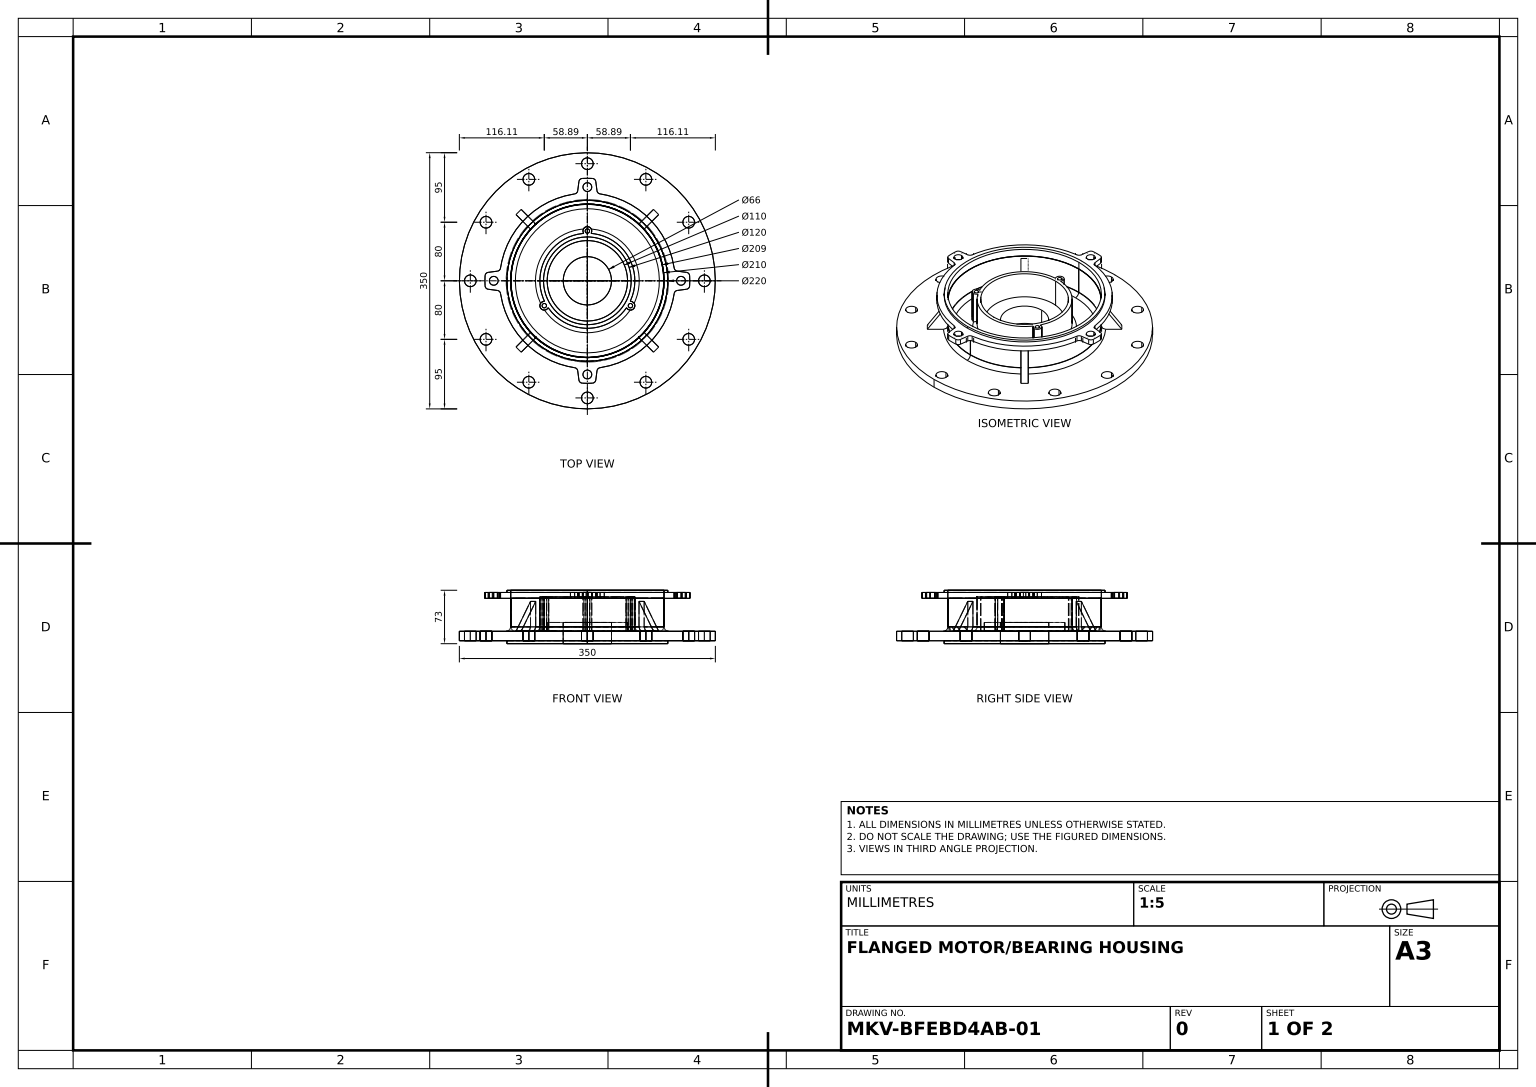
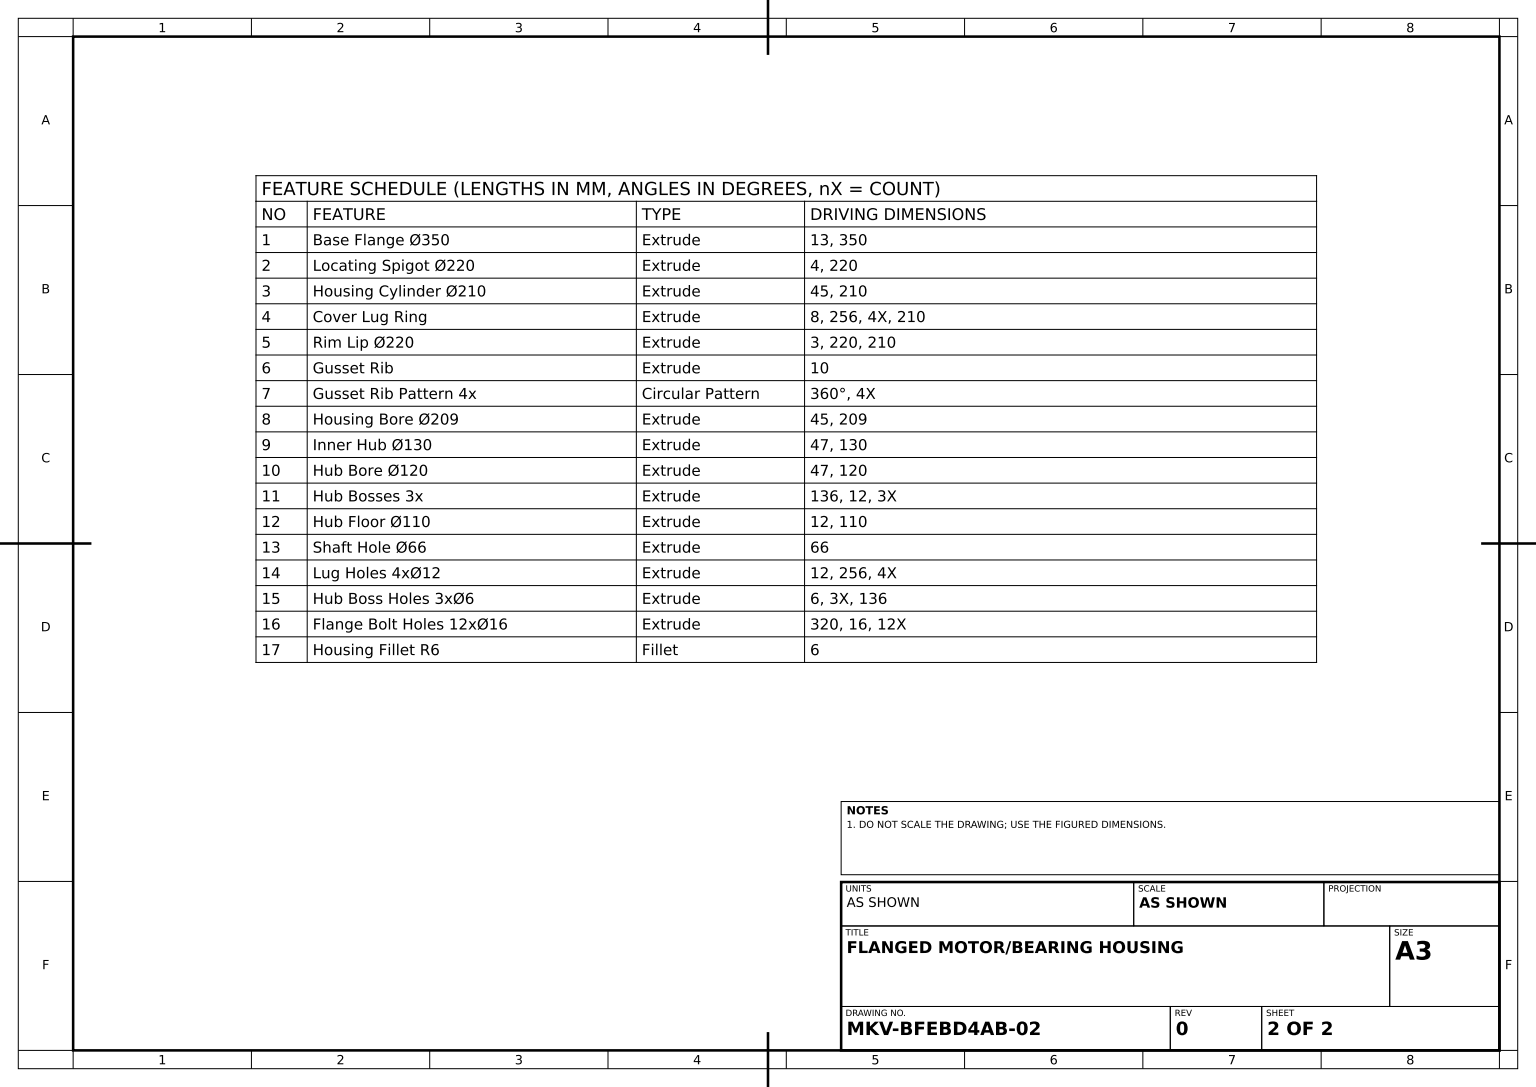
from build123d import *

# Parameters (mm, degrees)
FLANGE_SKETCH_350_R            = 175
BASE_FLANGE_350_DEPTH          = 13
SPIGOT_SKETCH_220_R            = 110
LOCATING_SPIGOT_220_DEPTH      = 4
HOUSING_SKETCH_210_R           = 105
HOUSING_CYLINDER_210_DEPTH     = 45
LUG_RING_SKETCH_R              = 105
COVER_LUG_RING_DEPTH           = 8
RIM_LIP_SKETCH_R               = 110
RIM_LIP_SKETCH_R_2             = 105
RIM_LIP_220_DEPTH              = 3
GUSSET_RIB_DEPTH               = 5
GUSSET_RIB_PATTERN_4X_COUNT    = 4
HOUSING_BORE_SKETCH_209_R      = 104.5
HOUSING_BORE_209_DEPTH         = 45
HUB_SKETCH_130_R               = 65
INNER_HUB_130_DEPTH            = 47
HUB_BORE_SKETCH_120_R          = 60
HUB_BORE_120_DEPTH             = 47
HUB_BOSSES_3X_REACH            = 257.629
HUB_BOSSES_SKETCH_3X_R         = 6
HUB_FLOOR_SKETCH_110_R         = 55
HUB_FLOOR_110_DEPTH            = 12
SHAFT_HOLE_SKETCH_66_R         = 33
SHAFT_HOLE_66_DEPTH            = 29
LUG_HOLES_SKETCH_4X_12_R       = 6
LUG_HOLES_4X_12_DEPTH          = 12
BOSS_HOLES_SKETCH_3X_6_R       = 3
HUB_BOSS_HOLES_3X_6_DEPTH      = 47
BOLT_HOLES_SKETCH_12X_16_R     = 8
FLANGE_BOLT_HOLES_12X_16_DEPTH = 13
HOUSING_FILLET_R6_R            = 6


with BuildPart() as part:
    # Flange Sketch Ø350 → Base Flange Ø350 (new body)
    with BuildSketch(Plane(origin=(0, 0, 0), x_dir=(1, 0, 0), z_dir=(0, 1, 0))):
        with Locations(Location((0, 0, 0), (0, 0, 90))):
            Circle(FLANGE_SKETCH_350_R)
    extrude(amount=BASE_FLANGE_350_DEPTH)

    # Spigot Sketch Ø220 → Locating Spigot Ø220 (add)
    with BuildSketch(Plane.XZ):
        with Locations(Location((0, 0, 0), (0, 0, 270))):
            Circle(SPIGOT_SKETCH_220_R)
    extrude(amount=LOCATING_SPIGOT_220_DEPTH)

    # Housing Sketch Ø210 → Housing Cylinder Ø210 (add)
    with BuildSketch(Plane(origin=(0, 13, 0), x_dir=(1, 0, 0), z_dir=(0, 1, 0))):
        with Locations(Location((0, 0, 0), (0, 0, 90))):
            Circle(HOUSING_SKETCH_210_R)
    extrude(amount=HOUSING_CYLINDER_210_DEPTH)

    # Gusset Rib Profile → Gusset Rib (add, symmetric)
    with BuildSketch(Plane(origin=(0, 0, 0), x_dir=(-0.707106781186549, 0, -0.7071067811865462), z_dir=(0.7071067811865462, 0, -0.707106781186549))):
        Polygon((102.938543902, 56.605912109), (102.938543902, 13), (132.938543902, 13), align=None)
    gusset_rib = extrude(amount=GUSSET_RIB_DEPTH, both=True)

    # Gusset Rib Pattern 4x: Gusset Rib ×4 about axis
    gusset_rib_pattern_4x_axis = Axis((0, 0, 0), (0, 1, 0))
    for i in range(1, GUSSET_RIB_PATTERN_4X_COUNT):
        add(gusset_rib.rotate(gusset_rib_pattern_4x_axis, i * 360 / GUSSET_RIB_PATTERN_4X_COUNT))

    # Housing Bore Sketch Ø209 → Housing Bore Ø209 (cut)
    with BuildSketch(Plane(origin=(0, 58, 0), x_dir=(1, 0, 0), z_dir=(0, 1, 0))):
        with Locations(Location((0, 0, 0), (0, 0, 270))):
            Circle(HOUSING_BORE_SKETCH_209_R)
    extrude(amount=-HOUSING_BORE_209_DEPTH, mode=Mode.SUBTRACT)

    # Hub Sketch Ø130 → Inner Hub Ø130 (add)
    with BuildSketch(Plane(origin=(0, 13, 0), x_dir=(1, 0, 0), z_dir=(0, 1, 0))):
        with Locations(Location((0, 0, 0), (0, 0, 270))):
            Circle(HUB_SKETCH_130_R)
    extrude(amount=INNER_HUB_130_DEPTH)

    # Hub Bore Sketch Ø120 → Hub Bore Ø120 (cut)
    with BuildSketch(Plane(origin=(0, 60, 0), x_dir=(1, 0, 0), z_dir=(0, 1, 0))):
        with Locations(Location((0, 0, 0), (0, 0, 270))):
            Circle(HUB_BORE_SKETCH_120_R)
    extrude(amount=-HUB_BORE_120_DEPTH, mode=Mode.SUBTRACT)

    # Hub Bosses Sketch 3x → Hub Bosses 3x (add, up to next)
    with BuildSketch(Plane(origin=(0, 60, 0), x_dir=(1, 0, 0), z_dir=(0, 1, 0)), mode=Mode.PRIVATE) as hub_bosses_3x_sk1:
        with Locations((0, 68)):
            Circle(HUB_BOSSES_SKETCH_3X_R)
    hub_bosses_3x_tool1 = extrude(hub_bosses_3x_sk1.sketch, amount=-HUB_BOSSES_3X_REACH, mode=Mode.PRIVATE) - part.part
    # Hub Bosses Sketch 3x → Hub Bosses 3x (add, up to next)
    with BuildSketch(Plane(origin=(0, 60, 0), x_dir=(1, 0, 0), z_dir=(0, 1, 0)), mode=Mode.PRIVATE) as hub_bosses_3x_sk2:
        with Locations((58.889727457, -34)):
            Circle(HUB_BOSSES_SKETCH_3X_R)
    hub_bosses_3x_tool2 = extrude(hub_bosses_3x_sk2.sketch, amount=-HUB_BOSSES_3X_REACH, mode=Mode.PRIVATE) - part.part
    # Hub Bosses Sketch 3x → Hub Bosses 3x (add, up to next)
    with BuildSketch(Plane(origin=(0, 60, 0), x_dir=(1, 0, 0), z_dir=(0, 1, 0)), mode=Mode.PRIVATE) as hub_bosses_3x_sk3:
        with Locations((-58.889727457, -34)):
            Circle(HUB_BOSSES_SKETCH_3X_R)
    hub_bosses_3x_tool3 = extrude(hub_bosses_3x_sk3.sketch, amount=-HUB_BOSSES_3X_REACH, mode=Mode.PRIVATE) - part.part
    add(hub_bosses_3x_tool1.solids().sort_by_distance((0, 60, -68))[0])
    add(hub_bosses_3x_tool2.solids().sort_by_distance((58.889727, 60, 34))[0])
    add(hub_bosses_3x_tool3.solids().sort_by_distance((-58.889727, 60, 34))[0])

    # Hub Floor Sketch Ø110 → Hub Floor Ø110 (add)
    with BuildSketch(Plane(origin=(0, 13, 0), x_dir=(1, 0, 0), z_dir=(0, 1, 0))):
        with Locations(Location((0, 0, 0), (0, 0, 270))):
            Circle(HUB_FLOOR_SKETCH_110_R)
    extrude(amount=HUB_FLOOR_110_DEPTH)

    # Shaft Hole Sketch Ø66 → Shaft Hole Ø66 (cut)
    with BuildSketch(Plane(origin=(0, 25, 0), x_dir=(1, 0, 0), z_dir=(0, 1, 0))):
        with Locations(Location((0, 0, 0), (0, 0, 270))):
            Circle(SHAFT_HOLE_SKETCH_66_R)
    extrude(amount=-SHAFT_HOLE_66_DEPTH, mode=Mode.SUBTRACT)

    # Boss Holes Sketch 3xØ6 → Hub Boss Holes 3xØ6 (cut)
    with BuildSketch(Plane(origin=(0, 60, 0), x_dir=(1, 0, 0), z_dir=(0, 1, 0))):
        with Locations(Location((0, 68, 0), (0, 0, 270))):
            Circle(BOSS_HOLES_SKETCH_3X_6_R)
        with Locations(Location((58.889727457, -34, 0), (0, 0, 270))):
            Circle(BOSS_HOLES_SKETCH_3X_6_R)
        with Locations(Location((-58.889727457, -34, 0), (0, 0, 270))):
            Circle(BOSS_HOLES_SKETCH_3X_6_R)
    extrude(amount=-HUB_BOSS_HOLES_3X_6_DEPTH, mode=Mode.SUBTRACT)

    # Bolt Holes Sketch 12xØ16 → Flange Bolt Holes 12xØ16 (cut)
    with BuildSketch(Plane(origin=(0, 13, 0), x_dir=(1, 0, 0), z_dir=(0, 1, 0))):
        with Locations(Location((0, 160, 0), (0, 0, 270))):
            Circle(BOLT_HOLES_SKETCH_12X_16_R)
        with Locations(Location((80, 138.564064606, 0), (0, 0, 270))):
            Circle(BOLT_HOLES_SKETCH_12X_16_R)
        with Locations(Location((138.564064606, 80, 0), (0, 0, 270))):
            Circle(BOLT_HOLES_SKETCH_12X_16_R)
        with Locations(Location((160, 0, 0), (0, 0, 270))):
            Circle(BOLT_HOLES_SKETCH_12X_16_R)
        with Locations(Location((138.564064606, -80, 0), (0, 0, 270))):
            Circle(BOLT_HOLES_SKETCH_12X_16_R)
        with Locations(Location((80, -138.564064606, 0), (0, 0, 270))):
            Circle(BOLT_HOLES_SKETCH_12X_16_R)
        with Locations(Location((0, -160, 0), (0, 0, 270))):
            Circle(BOLT_HOLES_SKETCH_12X_16_R)
        with Locations(Location((-80, -138.564064606, 0), (0, 0, 270))):
            Circle(BOLT_HOLES_SKETCH_12X_16_R)
        with Locations(Location((-138.564064606, -80, 0), (0, 0, 270))):
            Circle(BOLT_HOLES_SKETCH_12X_16_R)
        with Locations(Location((-160, 0, 0), (0, 0, 270))):
            Circle(BOLT_HOLES_SKETCH_12X_16_R)
        with Locations(Location((-138.564064606, 80, 0), (0, 0, 270))):
            Circle(BOLT_HOLES_SKETCH_12X_16_R)
        with Locations(Location((-80, 138.564064606, 0), (0, 0, 270))):
            Circle(BOLT_HOLES_SKETCH_12X_16_R)
    extrude(amount=-FLANGE_BOLT_HOLES_12X_16_DEPTH, mode=Mode.SUBTRACT)

    # Housing Fillet R6
    housing_fillet_r6_edges = [part.edges().sort_by_distance(p)[0] for p in [
        (56.291651246, 13, -32.5),
        (0, 13, 65),
        (-105, 13, 0),
        (0, 13, 105),
        (105, 13, 0),
        (-37.860008772, 13, -97.936815018),
        (0, 13, -104.5),
        (-56.291651246, 13, -32.5),
    ]]
    fillet(housing_fillet_r6_edges, radius=HOUSING_FILLET_R6_R)


with BuildPart() as body_2:
    # Lug Ring Sketch → Cover Lug Ring (new body)
    with BuildSketch(Plane(origin=(0, 58, 0), x_dir=(1, 0, 0), z_dir=(0, 1, 0))):
        with BuildLine():
            Line((135.492214872, 11.536480406), (123.024850581, 13.177840053))
            ThreePointArc((123.024850581, 13.177840053), (120.168019556, 14.573649393), (118.730382281, 17.409661786))
            ThreePointArc((118.730382281, 17.409661786), (84.852813742, 84.852813742), (17.409661786, 118.730382281))
            ThreePointArc((17.409661786, 118.730382281), (14.573649393, 120.168019556), (13.177840053, 123.024850581))
            Line((13.177840053, 123.024850581), (11.536480406, 135.492214872))
            ThreePointArc((11.536480406, 135.492214872), (9.96663562, 138.517308748), (6.822932251, 139.833642574))
            ThreePointArc((6.822932251, 139.833642574), (0, 140), (-6.822932251, 139.833642574))
            ThreePointArc((-6.822932251, 139.833642574), (-9.96663562, 138.517308748), (-11.536480406, 135.492214872))
            Line((-11.536480406, 135.492214872), (-13.177840053, 123.024850581))
            ThreePointArc((-13.177840053, 123.024850581), (-14.573649393, 120.168019556), (-17.409661786, 118.730382281))
            ThreePointArc((-17.409661786, 118.730382281), (-84.852813742, 84.852813742), (-118.730382281, 17.409661786))
            ThreePointArc((-118.730382281, 17.409661786), (-120.168019556, 14.573649393), (-123.024850581, 13.177840053))
            Line((-123.024850581, 13.177840053), (-135.492214872, 11.536480406))
            ThreePointArc((-135.492214872, 11.536480406), (-138.517308748, 9.96663562), (-139.833642574, 6.822932251))
            ThreePointArc((-139.833642574, 6.822932251), (-140, 0), (-139.833642574, -6.822932251))
            ThreePointArc((-139.833642574, -6.822932251), (-138.517308748, -9.96663562), (-135.492214872, -11.536480406))
            Line((-135.492214872, -11.536480406), (-123.024850581, -13.177840053))
            ThreePointArc((-123.024850581, -13.177840053), (-120.168019556, -14.573649393), (-118.730382281, -17.409661786))
            ThreePointArc((-118.730382281, -17.409661786), (-84.852813742, -84.852813742), (-17.409661786, -118.730382281))
            ThreePointArc((-17.409661786, -118.730382281), (-14.573649393, -120.168019556), (-13.177840053, -123.024850581))
            Line((-13.177840053, -123.024850581), (-11.536480406, -135.492214872))
            ThreePointArc((-11.536480406, -135.492214872), (-9.96663562, -138.517308748), (-6.822932251, -139.833642574))
            ThreePointArc((-6.822932251, -139.833642574), (0, -140), (6.822932251, -139.833642574))
            ThreePointArc((6.822932251, -139.833642574), (9.96663562, -138.517308748), (11.536480406, -135.492214872))
            Line((11.536480406, -135.492214872), (13.177840053, -123.024850581))
            ThreePointArc((13.177840053, -123.024850581), (14.573649393, -120.168019556), (17.409661786, -118.730382281))
            ThreePointArc((17.409661786, -118.730382281), (84.852813742, -84.852813742), (118.730382281, -17.409661786))
            ThreePointArc((118.730382281, -17.409661786), (120.168019556, -14.573649393), (123.024850581, -13.177840053))
            Line((123.024850581, -13.177840053), (135.492214872, -11.536480406))
            ThreePointArc((135.492214872, -11.536480406), (138.517308748, -9.96663562), (139.833642574, -6.822932251))
            ThreePointArc((139.833642574, -6.822932251), (140, 0), (139.833642574, 6.822932251))
            ThreePointArc((139.833642574, 6.822932251), (138.517308748, 9.96663562), (135.492214872, 11.536480406))
        make_face()
        with Locations(Location((0, 0, 0), (0, 0, 270))):
            Circle(LUG_RING_SKETCH_R, mode=Mode.SUBTRACT)
    extrude(amount=COVER_LUG_RING_DEPTH)

    # Rim Lip Sketch → Rim Lip Ø220 (add)
    with BuildSketch(Plane(origin=(0, 66, 0), x_dir=(1, 0, 0), z_dir=(0, 1, 0))):
        with Locations(Location((0, 0, 0), (0, 0, 90))):
            Circle(RIM_LIP_SKETCH_R)
        with Locations(Location((0, 0, 0), (0, 0, 270))):
            Circle(RIM_LIP_SKETCH_R_2, mode=Mode.SUBTRACT)
    extrude(amount=RIM_LIP_220_DEPTH)

    # Lug Holes Sketch 4xØ12 → Lug Holes 4xØ12 (cut)
    with BuildSketch(Plane(origin=(0, 66, 0), x_dir=(1, 0, 0), z_dir=(0, 1, 0))):
        with Locations(Location((0, 128, 0), (0, 0, 270))):
            Circle(LUG_HOLES_SKETCH_4X_12_R)
        with Locations(Location((128, 0, 0), (0, 0, 270))):
            Circle(LUG_HOLES_SKETCH_4X_12_R)
        with Locations(Location((0, -128, 0), (0, 0, 270))):
            Circle(LUG_HOLES_SKETCH_4X_12_R)
        with Locations(Location((-128, 0, 0), (0, 0, 270))):
            Circle(LUG_HOLES_SKETCH_4X_12_R)
    extrude(amount=-LUG_HOLES_4X_12_DEPTH, mode=Mode.SUBTRACT)


solid = Compound([part.part, body_2.part])
